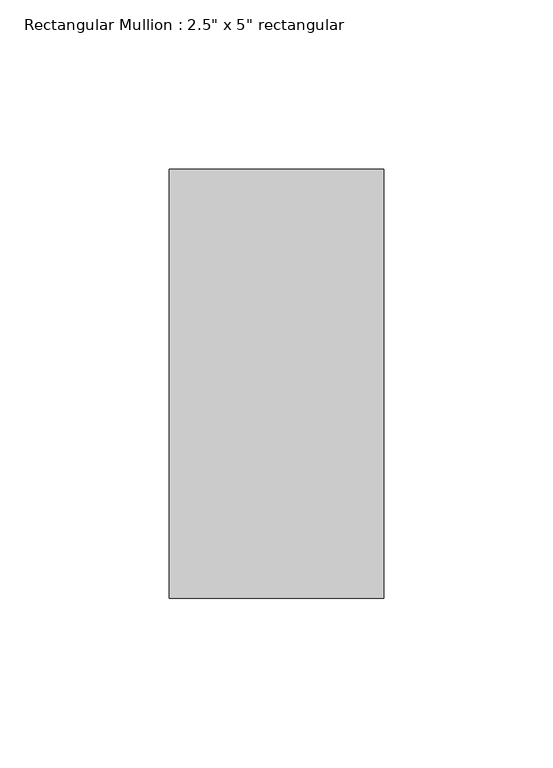
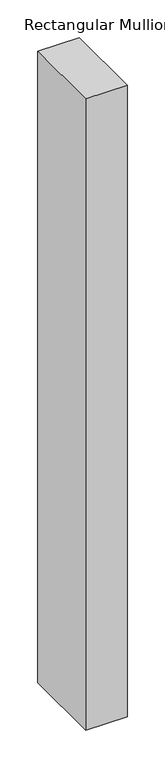
"""IFC4 building model written with IfcOpenShell, lengths in millimetres: member geometry."""

from ifc_helpers import new_model, si_unit, frame, origin, place, context, project, spatial, polyline, outline, extrude, source, transform, mapped, element, save


def member_38455fd9(model_context):
    return source(origin(), model_context, "Body", "SweptSolid", [
        extrude(outline(polyline([(31.75, 63.5), (31.75, -63.5), (-31.75, -63.5), (-31.75, 63.5), (31.75, 63.5)])), frame((0.0, 0.0, -1022.35), z_axis=(0.0, 0.0, 1.0), x_axis=(1.0, 0.0, 0.0)), (0.0, 0.0, 1.0), 1022.35),
    ])


if __name__ == "__main__":
    model = new_model("IFC4")
    model_context = context("Model", 3, world=origin())
    ifc_project = project(units=[si_unit("LENGTHUNIT", "METRE", prefix="MILLI")], contexts=[model_context])
    site = spatial("IfcSite", under=ifc_project)
    building = spatial("IfcBuilding", under=site)
    placement = place(None, origin())
    member_shape = member_38455fd9(model_context)
    element("IfcMember", 1, ObjectType="Rectangular Mullion : 2.5\" x 5\" rectangular", at=placement, inside=building, context=model_context, shape_type="MappedRepresentation", body=[
        mapped(member_shape, transform((0.0, 0.0, 0.0), x_axis=(1.0, 0.0, 0.0), y_axis=(0.0, 1.0, 0.0), z_axis=(0.0, 0.0, 1.0))),
    ])
    save(model, "model.ifc")

# Revit data of these elements
# Type "Rectangular Mullion : 2.5\" x 5\" rectangular"
#   built-in parameter 1007304 = 0.416667 (stored number, unit not read)
#   built-in parameter 1007301 = 0.104167 (stored number, unit not read)
#   built-in parameter 1007300 = 0.104167 (stored number, unit not read)
# Element 1 (IfcMember, "Rectangular Mullion : 2.5\" x 5\" rectangular")
#   Materials on its faces: "Aluminum"
# Materials
#   "Aluminum": class "Metal", colour RGB 247 247 247, transparency 0, Description = "Aluminum 6061", Cost = 0
